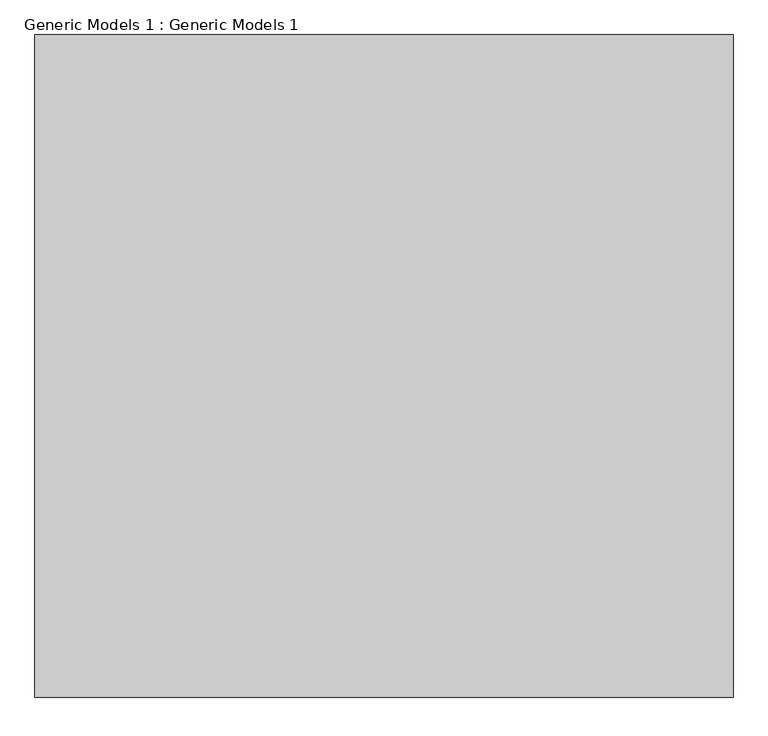
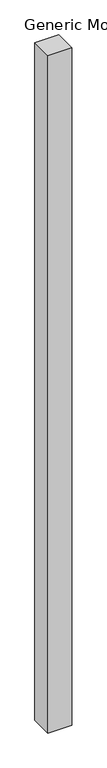
"""IFC4 building model written with IfcOpenShell, lengths in millimetres: proxy geometry, Generic Models 1 : Generic Models 1."""

from ifc_helpers import new_model, si_unit, origin, origin_with_axes, place, context, project, spatial, polyline, outline, extrude, source, transform, mapped, element, save


def generic_models_1_generic_models_1_ad90d225(model_context):
    return source(origin(), model_context, "Body", "SweptSolid", [
        extrude(outline(polyline([(8298.1159338, -14177.0998412), (6272.0794877, -14177.0998412), (6272.0794877, -12253.1237084), (8298.1159338, -12253.1237084), (8298.1159338, -14177.0998412)])), origin_with_axes(), (0.0, 0.0, 1.0), 60833.3935192),
    ])


if __name__ == "__main__":
    model = new_model("IFC4")
    model_context = context("Model", 3, world=origin())
    ifc_project = project(units=[si_unit("LENGTHUNIT", "METRE", prefix="MILLI")], contexts=[model_context])
    site = spatial("IfcSite", under=ifc_project)
    building = spatial("IfcBuilding", under=site)
    placement = place(None, origin())
    generic_models_1_generic_models_1_shape = generic_models_1_generic_models_1_ad90d225(model_context)
    element("IfcBuildingElementProxy", 1, Name="Generic Models 1 : Generic Models 1", ObjectType="Generic Models 1 : Generic Models 1", at=placement, inside=building, context=model_context, shape_type="MappedRepresentation", body=[
        mapped(generic_models_1_generic_models_1_shape, transform((0.0, 0.0, 0.0), x_axis=(1.0, 0.0, 0.0), y_axis=(0.0, 1.0, 0.0), z_axis=(0.0, 0.0, 1.0))),
    ])
    save(model, "model.ifc")
